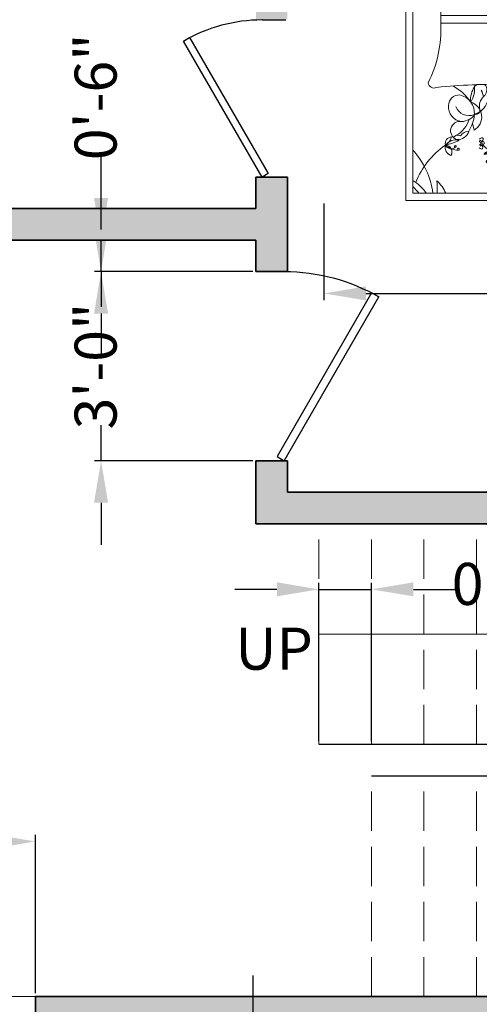
# Model space of a CAD drawing. Units: inches. Extents: x 2073 to 2646, y 2372 to 3017.
# Tile 5 of 8: x 2340 to 2428, y 2686 to 2874. Entities that reach past the tile are written whole.
import ezdxf

# ---------------------------------------------------------------- set-up
doc = ezdxf.new("R2010")
doc.units = ezdxf.units.IN
doc.linetypes.add('DASH', pattern=[0.35, 0.25, -0.1])
for name, color, linetype, lineweight in [('A-ANNO-DIMS', 2, 'Continuous', 18), ('A-ANNO-SYMB', 7, 'Continuous', 18), ('A-ANNO-TEXT', 7, 'Continuous', 25), ('A-DOOR', 3, 'Continuous', 25), ('A-FLOR-STRS', 7, 'Continuous', 25), ('A-FLOR-STRS-HIDN', 7, 'DASH', 18), ('A-FURN', 8, 'Continuous', 18), ('A-WALL', 7, 'Continuous', 35), ('A-WALL-OVHD', 7, 'DASH', 18), ('A-WALL-PATT', 30, 'Continuous', 13)]:
    doc.layers.add(name, color=color, linetype=linetype, lineweight=lineweight)
doc.styles.get("Standard").update_dxf_attribs({"font": 'arial.ttf'})
doc.dimstyles.new('ISO-25', dxfattribs={"dimtxt": 8, "dimasz": 8, "dimexe": 1.25, "dimexo": 0.625, "dimtad": 0, "dimdec": 1, "dimlunit": 4, "dimtxsty": 'Standard', "dimcen": 2.5, "dimadec": 0, "dimazin": 0, "dimtfac": 1, "dimtdec": 1, "dimtmove": 0, "dimatfit": 3, "dimfxl": 1, "dimarcsym": 0})

# ---------------------------------------------------------------- blocks, each defined once
blk = doc.blocks.new('bed')
at = {"color": 0}
for p, q in [((2249.53, 3172.75), (2367.64, 3172.75)), ((2273.15, 3172.75), (2273.15, 3140.33)), ((2261.34, 3155.19), (2261.34, 3170.62)), ((2344.02, 3171.23), (2273.15, 3171.23)), ((2355.83, 3155.19), (2355.83, 3170.62)), ((2269.06, 3162.9), (2253.62, 3162.9)), ((2348.11, 3162.9), (2363.55, 3162.9)), ((2273.15, 3154.08), (2344.02, 3154.08)), ((2289.56, 3150.57), (2302.44, 3154.08)), ((2305.6, 3154.08), (2299.13, 3145.07)), ((2280.95, 3147.46), (2289.56, 3150.57)), ((2343.7, 3149.18), (2301.65, 3148.59)), ((2276.4, 3144.12), (2280.95, 3147.46)), ((2343.66, 3147.96), (2300.77, 3147.36)), ((2272.09, 3139.1), (2276.4, 3144.12)), ((2299.13, 3145.07), (2296.5, 3138.14)), ((2343.59, 3144.24), (2298.75, 3144.07)), ((2343.6, 3143.03), (2298.28, 3142.85)), ((2273.05, 3138.14), (2272.09, 3139.1)), ((2277.84, 3138.62), (2273.05, 3138.14)), ((2283.82, 3138.14), (2277.84, 3138.62)), ((2289.08, 3137.42), (2283.82, 3138.14)), ((2296.5, 3138.14), (2296.02, 3135.03)), ((2292.19, 3135.99), (2289.08, 3137.42)), ((2296.02, 3135.03), (2292.19, 3135.99)), ((2265.12, 3114.85), (2271.8, 3114.85)), ((2265.12, 3072.3), (2265.12, 3114.85)), ((2344.68, 3114.85), (2351.23, 3114.85)), ((2351.23, 3114.85), (2351.23, 3072.3)), ((2271.8, 3113.48), (2266.49, 3113.48)), ((2266.49, 3113.48), (2266.49, 3073.67)), ((2349.86, 3113.48), (2344.65, 3113.48)), ((2349.86, 3073.67), (2349.86, 3113.48)), ((2344.56, 3107.48), (2271.79, 3107.48)), ((2344.67, 3106.01), (2271.79, 3106.01)), ((2332.56, 3094.41), (2284.61, 3094.41)), ((2278.13, 3085.65), (2277.87, 3086.98)), ((2286.38, 3085.65), (2286.64, 3086.98)), ((2329.96, 3085.65), (2329.7, 3086.98)), ((2338.22, 3085.65), (2338.48, 3086.98)), ((2266.49, 3073.67), (2349.86, 3073.67)), ((2351.23, 3072.3), (2265.12, 3072.3))]:
    blk.add_line(p, q, dxfattribs=at)
for points in [[(2273.15, 3153.06), (2249.53, 3153.06), (2249.53, 3172.75)], [(2344.02, 3172.75), (2344.02, 3153.06), (2367.64, 3153.06), (2367.64, 3172.75)], [(2261.34, 3162.9), (2262.72, 3165.29)], [(2355.83, 3162.9), (2354.45, 3165.29)], [(2261.34, 3162.9), (2262.72, 3160.52)], [(2355.83, 3162.9), (2354.45, 3160.52)]]:
    blk.add_lwpolyline(points, dxfattribs=at)
for points in [[(2279.94, 3169.8, 0.074897), (2280.08, 3162.09, -0.472817)], [(2337.23, 3169.8, -0.074897), (2337.09, 3162.09, 0.472817)], [(2308.03, 3161.66, 0.14099), (2308.27, 3169.53, 0.235245)], [(2313.08, 3161.66, -0.14099), (2312.84, 3169.53, -0.235245)], [(2271.85, 3128.28, 0.001242), (2271.79, 3105.87, -0.127202), (2269.42, 3094.7)], [(2344.52, 3108.41, 0.056112), (2345.38, 3101.91, 0.095341), (2347.04, 3095.66)]]:
    blk.add_lwpolyline(points, format="xyb", dxfattribs=at)
for centre, radius in [((2261.34, 3162.9), 5.51), ((2355.83, 3162.9), 5.51), ((2261.34, 3162.9), 2.76), ((2355.83, 3162.9), 2.76), ((2284.95, 3081.37), 0.301), ((2331.4, 3081.37), 0.301), ((2282.98, 3078.2), 0.301), ((2333.36, 3078.2), 0.301)]:
    blk.add_circle(centre, radius, dxfattribs=at)
for centre, radius, start, end in [((2345.04, 4293.82), 1125.9, 266.68521, 267.14978), ((2296.12, 3127.06), 42.84, 82.2196, 99.497), ((2323.22, 3149.14), 20.76, 76.3427, 101.1841), ((2272.13, 4293.82), 1125.9, 272.85022, 273.31479), ((2305.17, 3148.71), 21.05, 81.5249, 103.96), ((2314.46, 3163.91), 5.84, 63.3437, 106.1026), ((2294.98, 3158.99), 15.22, 155.1316, 191.7583), ((2322.19, 3158.99), 15.22, 348.2417, 24.8684), ((2294.11, 3157.71), 14.47, 354.0129, 15.8293), ((2327, 3157.71), 14.47, 164.1707, 185.9871), ((2284.15, 3171.19), 15.83, 255.1039, 281.0369), ((2292.48, 3182.44), 27.45, 258.0397, 289.2615), ((2303.6, 3176.44), 20.83, 259.8617, 283.6238), ((2315.25, 3161.88), 6.26, 245.0183, 288.5407), ((2326.19, 3170.02), 15.03, 243.8761, 286.1746), ((2333.02, 3171.19), 15.83, 258.9631, 284.8961), ((2555.75, 3139.65), 212.22, 176.1, 180.9282), ((2163.8, 3136.16), 108.33, 355.8294, 1.553), ((2274.12, 3180.92), 44.58, 267.4519, 281.3392), ((2284.77, 3127.79), 9.61, 66.2616, 101.3392), ((2304.22, 3179.66), 45.8, 250.1194, 259.3383), ((2620.36, 3131.93), 276.84, 179.1145, 184.8735), ((2295.75, 3134.94), 0.285, 268.8623, 19.7536), ((2346.15, 3095.06), 1.08, 246.5219, 33.8264), ((2270.51, 3094.78), 1.09, 183.98, 297.3412), ((2283.2, 2971.46), 122.95, 89.3433, 95.6887), ((2270.05, 3086.09), 8.94, 33.6671, 63.2997), ((2282.03, 3091.41), 4.56, 145.785, 184.7304), ((2273.33, 3093.53), 4.89, 328.8218, 9.1554), ((2279.39, 3093.1), 1.42, 120.0293, 142.325), ((2277.12, 3092.26), 3.76, 289.2822, 29.1751), ((2276.55, 3091.58), 3.4, 7.436, 29.9149), ((2278.79, 3093.38), 1.77, 311.5653, 23.8354), ((2279.39, 3093.1), 1.42, 44.4517, 63.558), ((2287.39, 3092.26), 3.76, 150.8249, 250.7178), ((2285.72, 3093.38), 1.77, 156.1646, 228.4347), ((2285.12, 3093.1), 1.42, 113.229, 135.5483), ((2287.96, 3091.58), 3.4, 150.0851, 172.564), ((2285.12, 3093.1), 1.42, 37.675, 66.7144), ((2282.48, 3091.41), 4.56, 355.2696, 34.215), ((2291.18, 3093.53), 4.89, 169.7133, 211.1782), ((2294.46, 3086.09), 8.94, 111.4941, 146.3329), ((2321.89, 3086.09), 8.94, 33.6671, 68.5059), ((2333.87, 3091.41), 4.56, 145.785, 184.7304), ((2325.17, 3093.53), 4.89, 328.8218, 10.2867), ((2331.23, 3093.1), 1.42, 113.2856, 142.325), ((2328.96, 3092.26), 3.76, 289.2822, 29.1751), ((2328.39, 3091.58), 3.4, 7.436, 29.9149), ((2331.23, 3093.1), 1.42, 44.4517, 66.7144), ((2330.63, 3093.38), 1.77, 311.5653, 23.8354), ((2336.18, 2979.53), 114.93, 85.2402, 91.8035), ((2339.23, 3092.26), 3.76, 150.8249, 250.7178), ((2337.56, 3093.38), 1.77, 156.1646, 228.4347), ((2336.96, 3093.1), 1.42, 106.6343, 135.5483), ((2339.8, 3091.58), 3.4, 150.0851, 172.564), ((2336.96, 3093.1), 1.42, 37.675, 72.5814), ((2334.32, 3091.41), 4.56, 355.2696, 34.215), ((2343.02, 3093.53), 4.89, 169.249, 211.1782), ((2346.3, 3086.09), 8.94, 113.6453, 146.3329), ((2275.26, 3090.38), 1.99, 84.4856, 181.0538), ((2274.65, 3088.91), 3.55, 355.2933, 76.921), ((2281.57, 3090.25), 2.42, 131.5653, 195.1471), ((2282.94, 3090.25), 2.42, 344.8529, 48.4347), ((2289.86, 3088.91), 3.55, 103.079, 184.7067), ((2289.25, 3090.38), 1.99, 358.9462, 95.5144), ((2327.09, 3090.38), 1.99, 84.4856, 181.0538), ((2326.48, 3088.91), 3.55, 355.2933, 76.921), ((2333.4, 3090.25), 2.42, 131.5653, 195.1471), ((2334.78, 3090.25), 2.42, 344.8529, 48.4347), ((2341.7, 3088.91), 3.55, 103.079, 184.7067), ((2341.09, 3090.38), 1.99, 358.9462, 95.5144), ((2276.08, 3090.1), 2.82, 174.9449, 262.8857), ((2277.18, 3091.17), 2.74, 201.5819, 291.4221), ((2276.66, 3088.19), 2.94, 299.9085, 73.1337), ((2278.52, 3089.43), 0.733, 257.3041, 15.1471), ((2287.85, 3088.19), 2.94, 106.8663, 240.0915), ((2285.99, 3089.43), 0.733, 164.8529, 282.6959), ((2287.32, 3091.17), 2.74, 248.5779, 338.4181), ((2288.43, 3090.1), 2.82, 277.1143, 5.0551), ((2327.91, 3090.1), 2.82, 174.9449, 262.8857), ((2329.02, 3091.17), 2.74, 201.5819, 291.4221), ((2328.5, 3088.19), 2.94, 299.9085, 73.1337), ((2330.36, 3089.43), 0.733, 257.3041, 15.1471), ((2339.68, 3088.19), 2.94, 106.8663, 240.0915), ((2337.82, 3089.43), 0.733, 164.8529, 282.6959), ((2339.16, 3091.17), 2.74, 248.5779, 338.4181), ((2340.27, 3090.1), 2.82, 277.1143, 5.0551), ((2275.43, 3085.55), 1.77, 80.264, 250.8688), ((2271.91, 3089.45), 5.58, 301.2614, 341.7045), ((2275.58, 3090.72), 3.43, 272.3591, 324.0401), ((2271.86, 3089), 6.34, 326.2883, 356.5076), ((2282.03, 3091.41), 4.56, 212.7011, 216.3445), ((2282.59, 3088.31), 0.228, 102.7051, 280.4384), ((2282.57, 3088.45), 0.37, 280.4384, 100.4136), ((2282.48, 3091.41), 4.56, 323.6555, 327.2989), ((2288.92, 3090.72), 3.43, 215.9599, 267.6409), ((2292.65, 3089), 6.34, 183.4924, 213.7117), ((2292.6, 3089.45), 5.58, 198.2955, 238.7386), ((2289.08, 3085.55), 1.77, 289.1312, 99.736), ((2309.53, 3086.61), 1.28, 63.0274, 163.8037), ((2308.24, 3089.6), 2.63, 271.4585, 315.3727), ((2310.75, 3086.61), 1.28, 16.1963, 116.9726), ((2312.05, 3089.6), 2.63, 224.6273, 268.5415), ((2327.26, 3085.55), 1.77, 80.264, 250.8688), ((2323.75, 3089.45), 5.58, 301.2614, 341.7045), ((2327.42, 3090.72), 3.43, 272.3591, 324.0401), ((2323.7, 3089), 6.34, 326.2883, 356.5076), ((2333.87, 3091.41), 4.56, 212.7011, 216.3445), ((2333.78, 3088.45), 0.37, 79.5864, 259.5616), ((2333.75, 3088.31), 0.228, 259.5616, 77.2949), ((2334.32, 3091.41), 4.56, 323.6555, 327.2989), ((2340.76, 3090.72), 3.43, 215.9599, 267.6409), ((2344.49, 3089), 6.34, 183.4924, 213.7117), ((2344.44, 3089.45), 5.58, 198.2955, 238.7386), ((2340.92, 3085.55), 1.77, 289.1312, 99.736), ((2275, 3086.08), 2.21, 265.969, 344.3045), ((2277.38, 3083.14), 2.36, 96.1662, 141.5825), ((2279.99, 3086.89), 1.9, 308.2101, 316.3071), ((2281.16, 3085.65), 0.567, 278.3432, 4.2869), ((2280.84, 3086.14), 0.99, 300.656, 332.6341), ((2281.59, 3085.49), 0.241, 55.7657, 157.4417), ((2290.78, 3082.37), 9.78, 153.0032, 159.8941), ((2281.96, 3085.71), 0.241, 84.3784, 186.0543), ((2281.74, 3086.68), 0.99, 269.1859, 301.164), ((2282.03, 3086.17), 0.567, 237.5332, 323.4768), ((2281.48, 3087.78), 1.9, 285.5129, 293.6099), ((2282.72, 3085.65), 0.62, 87.3579, 140.4944), ((2281.28, 3087.43), 1.87, 301.164, 321.5612), ((2279.77, 3087.76), 3.33, 324.6898, 333.4936), ((2287.12, 3083.14), 2.36, 38.4175, 83.8338), ((2289.51, 3086.08), 2.21, 195.6955, 274.031), ((2309.5, 3071.59), 15.42, 94.4623, 172.255), ((2309.57, 3085.82), 1.71, 137.7873, 219.1145), ((2307.63, 3085.87), 1.29, 298.5391, 58.3627), ((2309.31, 3084.75), 2.44, 45.5411, 114.3101), ((2311.53, 3097.27), 10.79, 252.593, 267.2582), ((2309.56, 3086.92), 1.26, 177.7585, 283.852), ((2311.99, 3088.23), 3.9, 198.9159, 238.011), ((2310.98, 3084.75), 2.44, 65.6899, 134.4589), ((2308.75, 3097.27), 10.79, 272.7418, 287.407), ((2309.83, 3085.86), 0.167, 283.852, 219.9245), ((2310.44, 3085.92), 0.101, 320.1909, 256.0209), ((2308.29, 3088.23), 3.9, 301.989, 341.0841), ((2310.72, 3086.92), 1.26, 256.148, 2.2415), ((2312.66, 3085.87), 1.29, 121.6373, 241.4609), ((2310.71, 3085.82), 1.71, 320.8855, 42.2127), ((2310.28, 3075.15), 11.94, 352.8636, 81.8197), ((2326.84, 3086.08), 2.21, 265.969, 344.3045), ((2329.22, 3083.14), 2.36, 96.1662, 141.5825), ((2335.06, 3087.43), 1.87, 218.4388, 238.836), ((2333.63, 3085.65), 0.62, 39.5056, 92.6421), ((2336.58, 3087.76), 3.33, 206.5064, 215.3102), ((2334.32, 3086.17), 0.567, 216.5232, 302.4668), ((2334.61, 3086.68), 0.99, 238.836, 270.8141), ((2334.87, 3087.78), 1.9, 246.3901, 254.4871), ((2325.57, 3082.37), 9.78, 20.1059, 26.9968), ((2334.38, 3085.71), 0.241, 353.9457, 95.6216), ((2334.76, 3085.49), 0.241, 22.5583, 124.2343), ((2335.19, 3085.65), 0.567, 175.7131, 261.6568), ((2335.5, 3086.14), 0.99, 207.3659, 239.344), ((2336.35, 3086.89), 1.9, 223.6929, 231.7899), ((2341.35, 3086.08), 2.21, 195.6955, 274.031), ((2338.96, 3083.14), 2.36, 38.4175, 83.8338), ((2273.92, 3083.1), 1.28, 92.9516, 193.728), ((2271.31, 3085.04), 2.63, 301.3827, 345.2969), ((2274.66, 3081.37), 2.44, 75.4653, 144.2343), ((2270.34, 3093.33), 10.79, 282.5173, 297.1824), ((2275.06, 3083.63), 1.09, 63.9755, 143.2681), ((2279.54, 3083.62), 0.502, 101.5637, 142.6358), ((2279.47, 3083.44), 0.287, 91.1081, 181.8675), ((2279.13, 3084.01), 0.723, 288.7263, 352.5032), ((2279.63, 3083.98), 0.232, 345.2356, 144.9248), ((2281.29, 3084.79), 0.62, 101.3256, 154.4621), ((2280.4, 3086.9), 1.87, 280.2588, 300.656), ((2280.83, 3088.39), 3.33, 268.3264, 277.1302), ((2290.78, 3082.37), 9.78, 163.5842, 183.8277), ((2289.45, 3083.63), 1.09, 36.7319, 116.0245), ((2289.85, 3081.37), 2.44, 35.7657, 104.5347), ((2294.17, 3093.33), 10.79, 242.8176, 257.4827), ((2290.59, 3083.1), 1.28, 346.272, 87.0484), ((2293.2, 3085.04), 2.63, 194.7031, 238.6173), ((2310.03, 3085.09), 0.192, 238.011, 71.5592), ((2310.06, 3085.18), 0.093, 71.5592, 188.0167), ((2310.25, 3085.09), 0.192, 108.4408, 301.989), ((2310.22, 3085.18), 0.093, 351.9833, 108.4408), ((2325.76, 3083.1), 1.28, 92.9516, 193.728), ((2323.15, 3085.04), 2.63, 301.3827, 345.2969), ((2326.5, 3081.37), 2.44, 75.4653, 144.2343), ((2322.18, 3093.33), 10.79, 282.5173, 297.1824), ((2326.9, 3083.63), 1.09, 63.9755, 143.2681), ((2325.57, 3082.37), 9.78, 356.1723, 16.4158), ((2335.95, 3086.9), 1.87, 239.344, 259.7412), ((2335.52, 3088.39), 3.33, 262.8698, 271.6736), ((2335.06, 3084.79), 0.62, 25.5379, 78.6744), ((2336.72, 3083.98), 0.232, 35.0752, 194.7644), ((2337.21, 3084.01), 0.723, 187.4968, 251.2737), ((2336.88, 3083.44), 0.287, 358.1325, 88.8919), ((2336.81, 3083.62), 0.502, 37.3642, 78.4363), ((2341.29, 3083.63), 1.09, 36.7319, 116.0245), ((2341.69, 3081.37), 2.44, 35.7657, 104.5347), ((2346, 3093.33), 10.79, 242.8176, 257.4827), ((2345.04, 3085.04), 2.63, 194.7031, 238.6173), ((2342.42, 3083.1), 1.28, 346.272, 87.0484), ((2255.01, 3071.59), 15.42, 7.745, 41.8856), ((2281.39, 3070.07), 15.42, 124.3865, 158.5908), ((2274.35, 3082.43), 1.71, 167.7115, 249.0387), ((2272.64, 3081.51), 1.29, 328.4633, 88.2869), ((2275.25, 3085.73), 3.9, 228.8402, 267.9352), ((2273.8, 3083.38), 1.26, 207.6827, 313.7762), ((2274.56, 3082.59), 0.167, 313.7762, 249.7183), ((2275.1, 3082.12), 0.093, 101.4834, 217.9409), ((2275.12, 3082.03), 0.192, 267.9352, 101.4834), ((2279.12, 3083.15), 0.301, 273.2768, 86.7232), ((2279.53, 3082.6), 0.497, 217.7621, 259.0403), ((2280.07, 3083.26), 0.913, 203.4276, 227.6104), ((2279.78, 3082.86), 0.622, 80.3487, 133.6538), ((2279.66, 3083.37), 0.492, 229.7889, 317.6792), ((2279.11, 3082.33), 0.699, 355.053, 68.3618), ((2279.66, 3082.21), 0.985, 83.0852, 105.7171), ((2279.58, 3082.29), 0.231, 232.4737, 355.053), ((2272.84, 3074.04), 11.21, 43.1541, 52.0459), ((2279.84, 3083.22), 0.259, 317.6792, 80.3487), ((2280.45, 3081.67), 0.567, 278.3432, 4.2869), ((2280.14, 3082.17), 0.99, 300.656, 332.6341), ((2280.88, 3081.52), 0.241, 55.7657, 157.4417), ((2285.91, 3082.12), 4.9, 184.756, 209.2041), ((2292.97, 3092.56), 16.14, 222.2412, 232.1744), ((2282.65, 3081.81), 1.37, 304.5369, 16.3699), ((2284.55, 3081.43), 0.97, 127.3105, 187.9252), ((2283.22, 3081.54), 0.996, 355.0106, 41.658), ((2284.62, 3081.78), 0.41, 126.1046, 271.4281), ((2284.57, 3081.9), 0.295, 353.7526, 131.7054), ((2284.3, 3081.55), 0.414, 0.0645, 61.1507), ((2284.39, 3081.9), 0.473, 311.8413, 355.7877), ((2285.37, 3081.83), 0.502, 101.5637, 176.365), ((2285.3, 3081.65), 0.287, 91.1081, 181.8675), ((2285.61, 3081.07), 0.622, 80.3487, 133.6538), ((2284.96, 3082.22), 0.723, 288.7263, 352.5032), ((2285.46, 3082.19), 0.232, 345.2356, 144.9248), ((2285.67, 3081.43), 0.259, 317.6792, 80.3487), ((2289.39, 3082.03), 0.192, 78.5166, 272.0648), ((2289.26, 3085.73), 3.9, 272.0648, 311.1598), ((2289.41, 3082.12), 0.093, 322.0591, 78.5166), ((2290.71, 3083.38), 1.26, 226.2238, 332.3173), ((2289.97, 3082.66), 0.101, 290.2667, 226.2271), ((2291.87, 3081.51), 1.29, 91.7131, 211.5367), ((2290.16, 3082.43), 1.71, 290.9613, 12.2885), ((2283.12, 3070.07), 15.42, 21.4092, 55.6135), ((2333.23, 3070.07), 15.42, 124.3865, 158.5908), ((2326.19, 3082.43), 1.71, 167.7115, 249.0387), ((2325.64, 3083.38), 1.26, 207.6827, 313.7762), ((2327.09, 3085.73), 3.9, 228.8402, 267.9352), ((2324.48, 3081.51), 1.29, 328.4633, 88.2869), ((2326.39, 3082.59), 0.167, 313.7762, 249.7183), ((2326.93, 3082.12), 0.093, 101.4834, 217.9409), ((2326.95, 3082.03), 0.192, 267.9352, 101.4834), ((2330.68, 3081.43), 0.259, 99.6513, 222.3208), ((2330.74, 3081.07), 0.622, 46.3462, 99.6513), ((2330.89, 3082.19), 0.232, 35.0752, 194.7644), ((2331.38, 3082.22), 0.723, 187.4968, 251.2737), ((2331.05, 3081.65), 0.287, 358.1325, 88.8919), ((2330.98, 3081.83), 0.502, 3.635, 78.4363), ((2331.77, 3081.9), 0.295, 48.2946, 186.2474), ((2331.95, 3081.9), 0.473, 184.2123, 228.1587), ((2332.05, 3081.55), 0.414, 118.8493, 179.9355), ((2331.73, 3081.78), 0.41, 268.5719, 53.8954), ((2333.13, 3081.54), 0.996, 138.342, 184.9894), ((2333.7, 3081.81), 1.37, 163.6301, 235.4631), ((2331.79, 3081.43), 0.97, 352.0748, 52.6895), ((2323.38, 3092.56), 16.14, 307.8256, 317.7588), ((2330.44, 3082.12), 4.9, 330.7959, 355.244), ((2343.51, 3074.04), 11.21, 127.9541, 136.8459), ((2335.46, 3081.52), 0.241, 22.5583, 124.2343), ((2335.89, 3081.67), 0.567, 175.7131, 261.6568), ((2336.21, 3082.17), 0.99, 207.3659, 239.344), ((2336.51, 3083.22), 0.259, 99.6513, 222.3208), ((2336.68, 3083.37), 0.492, 222.3208, 310.2111), ((2336.57, 3082.86), 0.622, 46.3462, 99.6513), ((2337.24, 3082.33), 0.699, 111.6382, 184.947), ((2336.77, 3082.29), 0.231, 184.947, 307.5263), ((2336.69, 3082.21), 0.985, 74.2829, 96.9148), ((2336.28, 3083.26), 0.913, 312.3896, 336.5724), ((2336.82, 3082.6), 0.497, 280.9597, 322.2379), ((2337.23, 3083.15), 0.301, 93.2768, 266.7232), ((2341.23, 3082.03), 0.192, 78.5166, 272.0648), ((2341.1, 3085.73), 3.9, 272.0648, 311.1598), ((2341.25, 3082.12), 0.093, 322.0591, 78.5166), ((2342.55, 3083.38), 1.26, 226.2238, 332.3173), ((2341.81, 3082.66), 0.101, 290.2667, 226.2271), ((2343.7, 3081.51), 1.29, 91.7131, 211.5367), ((2341.99, 3082.43), 1.71, 290.9613, 12.2885), ((2334.95, 3070.07), 15.42, 21.4092, 55.6135), ((2361.34, 3071.59), 15.42, 138.1144, 172.255), ((2280.59, 3080.82), 0.62, 101.3256, 154.4621), ((2279.69, 3082.92), 1.87, 280.2588, 300.656), ((2280.12, 3084.42), 3.33, 268.3264, 277.1302), ((2279.29, 3082.92), 1.9, 308.2101, 316.3071), ((2280.79, 3079.73), 0.336, 146.8636, 236.9021), ((2285.53, 3087.13), 8.79, 235.1882, 238.8844), ((2281.37, 3080.22), 0.909, 199.4799, 267.6828), ((2286.41, 3075.61), 5.88, 120.544, 139.818), ((2283.06, 3078.85), 0.97, 70.0041, 130.6188), ((2283.38, 3081.51), 0.833, 272.8499, 356.1226), ((2282.79, 3081.18), 0.807, 321.7607, 7.9252), ((2282.96, 3080.02), 0.807, 8.7227, 54.8872), ((2283, 3079.38), 1.37, 0.278, 72.111), ((2283.62, 3079.88), 0.833, 20.5253, 88.5375), ((2284.72, 3080.29), 0.97, 188.7227, 249.3375), ((2284.32, 3080.8), 0.298, 148.0499, 225.6268), ((2286.41, 3075.61), 5.88, 113.0501, 113.8477), ((2284.87, 3080.46), 0.948, 104.7558, 148.0499), ((2284.34, 3081.14), 0.594, 247.4086, 351.4386), ((2283.47, 3079.81), 0.996, 334.9899, 21.6373), ((2284.51, 3081.11), 0.199, 262.906, 7.132), ((2285.36, 3080.81), 0.497, 151.2196, 259.0403), ((2285.9, 3081.47), 0.913, 203.4276, 227.6104), ((2285.5, 3081.59), 0.492, 229.7889, 317.6792), ((2284.94, 3080.54), 0.699, 355.053, 68.3618), ((2285.49, 3080.43), 0.985, 83.0852, 105.7171), ((2285.41, 3080.5), 0.231, 232.4737, 355.053), ((2286.41, 3075.61), 5.88, 87.1071, 94.7585), ((2329.94, 3075.61), 5.88, 85.2415, 92.8929), ((2330.85, 3081.59), 0.492, 222.3208, 310.2111), ((2331.41, 3080.54), 0.699, 111.6382, 184.947), ((2330.94, 3080.5), 0.231, 184.947, 307.5263), ((2330.86, 3080.43), 0.985, 74.2829, 96.9148), ((2330.45, 3081.47), 0.913, 312.3896, 336.5724), ((2330.99, 3080.81), 0.497, 280.9597, 28.7804), ((2332.01, 3081.14), 0.594, 188.5614, 292.5914), ((2331.84, 3081.11), 0.199, 172.868, 277.094), ((2331.48, 3080.46), 0.948, 31.9501, 75.2442), ((2332.87, 3079.81), 0.996, 158.3627, 205.0101), ((2332.73, 3079.88), 0.833, 91.4625, 159.4747), ((2333.34, 3079.38), 1.37, 107.889, 179.722), ((2331.63, 3080.29), 0.97, 290.6625, 351.2773), ((2332.97, 3081.51), 0.833, 183.8774, 267.1501), ((2329.94, 3075.61), 5.88, 66.1523, 66.9499), ((2332.03, 3080.8), 0.298, 314.3732, 31.9501), ((2333.39, 3080.02), 0.807, 125.1128, 171.2773), ((2333.55, 3081.18), 0.807, 172.0748, 218.2393), ((2329.94, 3075.61), 5.88, 40.182, 59.456), ((2333.29, 3078.85), 0.97, 49.3812, 109.9959), ((2334.98, 3080.22), 0.909, 272.3172, 340.5201), ((2330.82, 3087.13), 8.79, 301.1156, 304.8118), ((2337.06, 3082.92), 1.9, 223.6929, 231.7899), ((2336.65, 3082.92), 1.87, 239.344, 259.7412), ((2335.55, 3079.73), 0.336, 303.0979, 33.1364), ((2336.22, 3084.42), 3.33, 262.8698, 271.6736), ((2335.76, 3080.82), 0.62, 25.5379, 78.6744), ((2281.27, 3079.88), 0.783, 212.8155, 277.3992), ((2280.81, 3079.35), 0.909, 266.9701, 338.2913), ((2276.02, 3085.84), 8.79, 302.6784, 306.3746), ((2281.04, 3078.63), 0.336, 214.3538, 304.3923), ((2281.17, 3079.91), 0.348, 238.8844, 314.2646), ((2281.09, 3079.13), 0.783, 280.3057, 17.1958), ((2281.03, 3079.05), 0.348, 306.3746, 21.7548), ((2281.59, 3079.27), 0.262, 19.3605, 201.7548), ((2281.59, 3079.47), 0.262, 311.8703, 134.2646), ((2286.53, 3077.08), 5.24, 153.7819, 158.2913), ((2282.36, 3080.66), 1.37, 247.2305, 319.0635), ((2281.9, 3080.2), 0.807, 264.4544, 310.6188), ((2285.91, 3082.12), 4.9, 214.0033, 222.4917), ((2282.49, 3079.88), 0.833, 218.3208, 298.8162), ((2282.9, 3077.29), 0.948, 104.7558, 148.0499), ((2282.65, 3078.61), 0.41, 126.1046, 271.4281), ((2282.61, 3078.72), 0.295, 353.7526, 131.7054), ((2282.54, 3077.94), 0.199, 262.906, 7.132), ((2282.33, 3078.37), 0.414, 0.0645, 61.1507), ((2282.43, 3078.73), 0.473, 311.8413, 355.7877), ((2282.43, 3080.03), 0.996, 297.7043, 344.3516), ((2283.4, 3078.66), 0.502, 101.5637, 176.365), ((2283.33, 3078.48), 0.287, 91.1081, 181.8675), ((2283.93, 3078.3), 0.913, 203.4276, 227.6104), ((2283.64, 3077.9), 0.622, 80.3487, 133.6538), ((2283.53, 3078.42), 0.492, 229.7889, 317.6792), ((2283, 3079.05), 0.723, 288.7263, 352.5032), ((2282.97, 3077.37), 0.699, 355.053, 68.3618), ((2283.52, 3077.26), 0.985, 83.0852, 105.7171), ((2283.49, 3079.02), 0.232, 345.2356, 144.9248), ((2283.7, 3078.26), 0.259, 317.6792, 80.3487), ((2308.32, 3063.33), 15.42, 94.4623, 117.4146), ((2308.39, 3077.56), 1.71, 137.7873, 219.1145), ((2306.45, 3077.61), 1.29, 298.5391, 58.3627), ((2308.35, 3078.35), 1.28, 63.0274, 163.8037), ((2307.06, 3081.34), 2.63, 271.4585, 315.3727), ((2308.13, 3076.49), 2.44, 45.5411, 114.3101), ((2310.81, 3079.97), 3.9, 198.9159, 238.011), ((2310.35, 3089), 10.79, 252.593, 267.2582), ((2308.38, 3078.66), 1.26, 177.7585, 283.852), ((2312.16, 3076.49), 2.44, 65.6899, 134.4589), ((2309.93, 3089), 10.79, 272.7418, 287.407), ((2311.93, 3078.35), 1.28, 16.1963, 116.9726), ((2313.23, 3081.34), 2.63, 224.6273, 268.5415), ((2309.47, 3079.97), 3.9, 301.989, 341.0841), ((2311.9, 3078.66), 1.26, 256.148, 2.2415), ((2313.84, 3077.61), 1.29, 121.6373, 241.4609), ((2311.89, 3077.56), 1.71, 320.8855, 42.2127), ((2311.96, 3063.33), 15.42, 62.5854, 85.5377), ((2332.65, 3078.26), 0.259, 99.6513, 222.3208), ((2332.82, 3078.42), 0.492, 222.3208, 310.2111), ((2332.71, 3077.9), 0.622, 46.3462, 99.6513), ((2332.86, 3079.02), 0.232, 35.0752, 194.7644), ((2333.35, 3079.05), 0.723, 187.4968, 251.2737), ((2333.37, 3077.37), 0.699, 111.6382, 184.947), ((2332.83, 3077.26), 0.985, 74.2829, 96.9148), ((2333.99, 3080.66), 1.37, 220.9365, 292.7695), ((2333.91, 3080.03), 0.996, 195.6484, 242.2957), ((2333.01, 3078.48), 0.287, 358.1325, 88.8919), ((2332.42, 3078.3), 0.913, 312.3896, 336.5724), ((2332.95, 3078.66), 0.502, 3.635, 78.4363), ((2333.85, 3079.88), 0.833, 241.1838, 321.6792), ((2333.74, 3078.72), 0.295, 48.2946, 186.2474), ((2333.92, 3078.73), 0.473, 184.2123, 228.1587), ((2334.02, 3078.37), 0.414, 118.8493, 179.9355), ((2333.81, 3077.94), 0.199, 172.868, 277.094), ((2333.7, 3078.61), 0.41, 268.5719, 53.8954), ((2333.44, 3077.29), 0.948, 31.9501, 75.2442), ((2334.44, 3080.2), 0.807, 229.3812, 275.5456), ((2330.44, 3082.12), 4.9, 317.5083, 325.9967), ((2335.25, 3079.13), 0.783, 162.8042, 259.6943), ((2334.75, 3079.47), 0.262, 45.7354, 228.1297), ((2334.75, 3079.27), 0.262, 338.2452, 160.6395), ((2329.82, 3077.08), 5.24, 21.7087, 26.2181), ((2335.53, 3079.35), 0.909, 201.7087, 273.0299), ((2335.18, 3079.91), 0.348, 225.7354, 301.1156), ((2335.32, 3079.05), 0.348, 158.2452, 233.6254), ((2335.08, 3079.88), 0.783, 262.6008, 327.1845), ((2340.32, 3085.84), 8.79, 233.6254, 237.3216), ((2335.3, 3078.63), 0.336, 235.6077, 325.6462), ((2282.35, 3077.63), 0.298, 148.0499, 225.6268), ((2282.37, 3077.97), 0.594, 247.4086, 351.4386), ((2283.39, 3077.64), 0.497, 151.2196, 259.0403), ((2283.44, 3077.33), 0.231, 232.4737, 355.053), ((2301.77, 3069.53), 7.52, 91.272, 146.5383), ((2304.47, 3068.13), 9.37, 107.8504, 143.6964), ((2309.39, 3065.49), 13.93, 124.0123, 144.053), ((2308.65, 3077.6), 0.167, 283.852, 219.9245), ((2308.85, 3076.83), 0.192, 238.011, 71.5592), ((2308.88, 3076.92), 0.093, 71.5592, 188.0167), ((2311.44, 3076.83), 0.192, 108.4408, 301.989), ((2311.4, 3076.92), 0.093, 351.9833, 108.4408), ((2311.62, 3077.66), 0.101, 320.1909, 256.0209), ((2311.82, 3076.24), 6.91, 338.117, 6.6195), ((2318.16, 3074.32), 2.77, 346.3898, 79.0739), ((2316.08, 3074.7), 3.5, 342.8609, 41.9049), ((2332.91, 3077.33), 0.231, 184.947, 307.5263), ((2332.95, 3077.64), 0.497, 280.9597, 28.7804), ((2333.98, 3077.97), 0.594, 188.5614, 292.5914), ((2334, 3077.63), 0.298, 314.3732, 31.9501), ((2262.74, 3069.53), 7.52, 33.4617, 60.1116), ((2260.04, 3068.13), 9.37, 36.3036, 46.4814), ((2266.95, 3071.27), 6.27, 22.5547, 48.9546), ((2249.77, 3074.64), 21.34, 357.4081, 3.6519), ((2297.56, 3071.27), 6.27, 131.0454, 157.4453), ((2314.73, 3074.64), 21.34, 176.3481, 182.5919), ((2301.61, 3074.64), 21.34, 357.4081, 3.6519), ((2318.79, 3071.27), 6.27, 22.5547, 48.9546), ((2349.39, 3071.27), 6.27, 131.0454, 157.4453), ((2366.57, 3074.64), 21.34, 176.3481, 182.5919), ((2353.6, 3069.53), 7.52, 119.8884, 146.5383), ((2356.31, 3068.13), 9.37, 133.5186, 143.6964), ((2304.01, 3065.56), 8.48, 73.5431, 107.0202), ((2307.37, 3061.19), 12.54, 94.3787, 95.6357), ((2313.97, 3052.6), 22.41, 109.7217, 109.9028), ((2316.27, 3065.56), 8.48, 72.9798, 106.4569), ((2312.91, 3061.19), 12.54, 84.3643, 85.6213), ((2306.31, 3052.6), 22.41, 70.0972, 70.2783)]:
    blk.add_arc(centre, radius, start, end, dxfattribs=at)
blk = doc.blocks.new('*U19')
for p, q in [((0, 0), (0, -6)), ((40, 0), (40, -6))]:
    blk.add_line(p, q)
blk.add_lwpolyline([(0, 0), (34.64, 20), (35.52, 18.48), (0.87, -1.52)], close=True)
blk.add_arc((0, 0), 40, 0, 30)
blk = doc.blocks.new('*D35')
at = {"layer": 'A-ANNO-DIMS', "color": 0, "lineweight": -2, "transparency": 16777216}
for p, q in [((2398.23, 2838.6), (2398.23, 2820.25)), ((2516.35, 2838.6), (2516.35, 2820.25)), ((2406.23, 2821.5), (2508.35, 2821.5)), ((2516.35, 2821.5), (2524.35, 2821.5))]:
    blk.add_line(p, q, dxfattribs=at)
at = {"layer": 'A-ANNO-DIMS', "color": 0, "transparency": 16777216}
for points in [[(2406.23, 2822.84), (2406.23, 2820.17), (2398.23, 2821.5)], [(2508.35, 2822.84), (2508.35, 2820.17), (2516.35, 2821.5)]]:
    blk.add_solid(points, dxfattribs=at)
at = {"layer": 'Defpoints', "color": 0, "transparency": 16777216}
for p in [(2398.23, 2839.22), (2516.35, 2839.22), (2516.35, 2821.5)]:
    blk.add_point(p, dxfattribs=at)
at = {"layer": 'A-ANNO-DIMS', "color": 0, "transparency": 16777216, "insert": (2587.37, 2821.5), "char_height": 8, "attachment_point": 5}
blk.add_mtext('BED GROUP 9\'-10" TYP.', dxfattribs=at)
blk = doc.blocks.new('*D50')
at = {"layer": 'A-ANNO-DIMS', "color": 0, "lineweight": -2, "transparency": 16777216}
for p, q in [((2355.79, 2833.66), (2355.79, 2841.66)), ((2384.67, 2825.66), (2354.54, 2825.66)), ((2355.79, 2825.66), (2355.79, 2818.92)), ((2355.79, 2789.66), (2355.79, 2796.41)), ((2384.67, 2789.66), (2354.54, 2789.66)), ((2355.79, 2781.66), (2355.79, 2773.66))]:
    blk.add_line(p, q, dxfattribs=at)
at = {"layer": 'A-ANNO-DIMS', "color": 0, "transparency": 16777216}
for points in [[(2354.46, 2833.66), (2357.12, 2833.66), (2355.79, 2825.66)], [(2354.46, 2781.66), (2357.12, 2781.66), (2355.79, 2789.66)]]:
    blk.add_solid(points, dxfattribs=at)
at = {"layer": 'Defpoints', "color": 0, "transparency": 16777216}
for p in [(2355.79, 2825.66), (2385.29, 2825.66), (2385.29, 2789.66)]:
    blk.add_point(p, dxfattribs=at)
at = {"layer": 'A-ANNO-DIMS', "color": 0, "transparency": 16777216, "insert": (2355.79, 2807.66), "char_height": 8, "attachment_point": 5, "rotation": 90}
blk.add_mtext('3\'-0"', dxfattribs=at)
blk = doc.blocks.new('*D52')
at = {"layer": 'A-ANNO-DIMS', "color": 0, "lineweight": -2, "transparency": 16777216}
for p, q in [((2283.29, 2688.29), (2283.29, 2718.41)), ((2343.29, 2688.29), (2343.29, 2718.41)), ((2291.29, 2717.16), (2302.03, 2717.16)), ((2335.29, 2717.16), (2324.55, 2717.16))]:
    blk.add_line(p, q, dxfattribs=at)
at = {"layer": 'A-ANNO-DIMS', "color": 0, "transparency": 16777216}
for points in [[(2291.29, 2718.5), (2291.29, 2715.83), (2283.29, 2717.16)], [(2335.29, 2718.5), (2335.29, 2715.83), (2343.29, 2717.16)]]:
    blk.add_solid(points, dxfattribs=at)
at = {"layer": 'Defpoints', "color": 0, "transparency": 16777216}
for p in [(2343.29, 2717.16), (2283.29, 2687.66), (2343.29, 2687.66)]:
    blk.add_point(p, dxfattribs=at)
at = {"layer": 'A-ANNO-DIMS', "color": 0, "transparency": 16777216, "insert": (2313.29, 2717.16), "char_height": 8, "attachment_point": 5}
blk.add_mtext('5\'-0"', dxfattribs=at)
blk = doc.blocks.new('*D53')
at = {"layer": 'A-ANNO-DIMS', "color": 0, "lineweight": -2, "transparency": 16777216}
for p, q in [((2384.79, 2683.66), (2384.79, 2691.66)), ((2355.92, 2675.66), (2386.04, 2675.66)), ((2384.79, 2675.66), (2384.79, 2668.92)), ((2384.79, 2639.66), (2384.79, 2646.41)), ((2355.92, 2639.66), (2386.04, 2639.66)), ((2384.79, 2631.66), (2384.79, 2623.66))]:
    blk.add_line(p, q, dxfattribs=at)
at = {"layer": 'A-ANNO-DIMS', "color": 0, "transparency": 16777216}
for points in [[(2383.46, 2683.66), (2386.12, 2683.66), (2384.79, 2675.66)], [(2383.46, 2631.66), (2386.12, 2631.66), (2384.79, 2639.66)]]:
    blk.add_solid(points, dxfattribs=at)
at = {"layer": 'Defpoints', "color": 0, "transparency": 16777216}
for p in [(2355.29, 2675.66), (2355.29, 2639.66), (2384.79, 2639.66)]:
    blk.add_point(p, dxfattribs=at)
at = {"layer": 'A-ANNO-DIMS', "color": 0, "transparency": 16777216, "insert": (2384.79, 2657.66), "char_height": 8, "attachment_point": 5, "rotation": 90}
blk.add_mtext('3\'-0"', dxfattribs=at)
blk = doc.blocks.new('*D67')
at = {"layer": 'A-ANNO-DIMS', "color": 0, "lineweight": -2, "transparency": 16777216}
for p, q in [((2389.29, 2765.16), (2381.29, 2765.16)), ((2397.29, 2736.29), (2397.29, 2766.41)), ((2397.29, 2765.16), (2407.29, 2765.16)), ((2407.29, 2736.29), (2407.29, 2766.41)), ((2415.29, 2765.16), (2423.29, 2765.16))]:
    blk.add_line(p, q, dxfattribs=at)
at = {"layer": 'A-ANNO-DIMS', "color": 0, "transparency": 16777216}
for points in [[(2389.29, 2766.5), (2389.29, 2763.83), (2397.29, 2765.16)], [(2415.29, 2766.5), (2415.29, 2763.83), (2407.29, 2765.16)]]:
    blk.add_solid(points, dxfattribs=at)
at = {"layer": 'Defpoints', "color": 0, "transparency": 16777216}
for p in [(2407.29, 2765.16), (2397.29, 2735.66), (2407.29, 2735.66)]:
    blk.add_point(p, dxfattribs=at)
at = {"layer": 'A-ANNO-DIMS', "color": 0, "transparency": 16777216, "insert": (2437.66, 2765.16), "char_height": 8, "attachment_point": 5}
blk.add_mtext('0\'-10"', dxfattribs=at)
blk = doc.blocks.new('*D70')
at = {"layer": 'A-ANNO-DIMS', "color": 0, "lineweight": -2, "transparency": 16777216}
for p, q in [((2355.79, 2839.66), (2355.79, 2847.66)), ((2384.67, 2831.66), (2354.54, 2831.66)), ((2355.79, 2825.66), (2355.79, 2831.66)), ((2384.67, 2825.66), (2354.54, 2825.66)), ((2355.79, 2817.66), (2355.79, 2809.66))]:
    blk.add_line(p, q, dxfattribs=at)
at = {"layer": 'A-ANNO-DIMS', "color": 0, "transparency": 16777216}
for points in [[(2354.46, 2839.66), (2357.12, 2839.66), (2355.79, 2831.66)], [(2354.46, 2817.66), (2357.12, 2817.66), (2355.79, 2825.66)]]:
    blk.add_solid(points, dxfattribs=at)
at = {"layer": 'Defpoints', "color": 0, "transparency": 16777216}
for p in [(2355.79, 2831.66), (2385.29, 2831.66), (2385.29, 2825.66)]:
    blk.add_point(p, dxfattribs=at)
at = {"layer": 'A-ANNO-DIMS', "color": 0, "transparency": 16777216, "insert": (2355.79, 2858.92), "char_height": 8, "attachment_point": 5, "rotation": 90}
blk.add_mtext('0\'-6"', dxfattribs=at)

msp = doc.modelspace()

# ---------------------------------------------------------------- hatches: boundary and pattern name
at = {"layer": 'A-WALL-PATT'}
h = msp.add_hatch(color=256, dxfattribs=at)
h.dxf.hatch_style = 1
h.paths.add_polyline_path([(2340.29, 2948.66), (2148.29, 2948.66), (2148.29, 2924.66), (2157.29, 2924.66), (2157.29, 2939.66), (2313.29, 2939.66), (2313.29, 2885.66), (2307.29, 2885.66), (2307.29, 2879.66), (2313.29, 2879.66), (2313.29, 2777.66), (2319.29, 2777.66), (2319.29, 2831.66), (2385.29, 2831.66), (2385.29, 2825.68), (2390.69, 2825.68, -0.004149), (2391.29, 2825.68), (2391.29, 2843.66), (2385.29, 2843.66), (2385.29, 2837.66), (2319.29, 2837.66), (2319.29, 2939.66), (2340.29, 2939.66)])
h.paths.add_polyline_path([(2271.29, 2885.66), (2157.29, 2885.66), (2157.29, 2900.66), (2148.29, 2900.66), (2148.29, 2856.74), (2157.29, 2856.74), (2157.29, 2879.66), (2271.29, 2879.66)], flags=17)
h.paths.add_polyline_path([(2157.29, 2796.74), (2148.29, 2796.74), (2148.29, 2764.25), (2157.29, 2764.25)])
h.paths.add_polyline_path([(2157.29, 2681.66), (2283.29, 2681.66), (2283.29, 2687.66), (2157.29, 2687.66), (2157.29, 2704.25), (2148.29, 2704.25), (2148.29, 2621.66), (2157.29, 2621.66)])
h.paths.add_polyline_path([(2196.29, 2501.66), (2157.29, 2501.66), (2157.29, 2561.66), (2148.29, 2561.66), (2148.29, 2492.66), (2196.29, 2492.66)])
h.paths.add_polyline_path([(2295.23, 2495.54), (2295.23, 2501.66), (2256.29, 2501.66), (2256.29, 2492.66), (2295.23, 2492.66)])
h.paths.add_polyline_path([(2355.29, 2603.66), (2361.29, 2603.66), (2361.29, 2609.66), (2355.29, 2609.66), (2355.29, 2639.66), (2349.29, 2639.66), (2349.29, 2501.66), (2343.29, 2501.66), (2343.29, 2492.66), (2349.29, 2492.66), (2349.29, 2420.66), (2532.29, 2420.66), (2532.29, 2486.66), (2523.29, 2486.66), (2523.29, 2429.66), (2355.29, 2429.66)])
h.paths.add_polyline_path([(2532.29, 2633.66), (2523.29, 2633.66), (2523.29, 2609.66), (2439.29, 2609.66), (2439.29, 2615.66), (2433.29, 2615.66), (2433.29, 2609.66), (2397.31, 2609.66), (2397.31, 2604.26, -0.004149), (2397.3, 2603.66), (2523.29, 2603.66), (2523.29, 2546.66), (2532.29, 2546.66)], flags=17)
h.paths.add_polyline_path([(2532.29, 2702.66), (2523.29, 2702.66), (2523.29, 2687.66), (2385.29, 2687.66), (2343.29, 2687.66), (2343.29, 2681.66), (2349.29, 2681.66), (2349.29, 2675.66), (2355.29, 2675.66), (2355.29, 2681.66), (2433.29, 2681.66), (2433.29, 2645.66), (2439.29, 2645.66), (2439.29, 2681.66), (2523.29, 2681.66), (2523.29, 2657.66), (2532.29, 2657.66)])
h.paths.add_polyline_path([(2532.29, 2831.66), (2523.29, 2831.66), (2523.29, 2783.66), (2391.29, 2783.66), (2391.29, 2789.66), (2385.29, 2789.66), (2385.29, 2777.66), (2523.29, 2777.66), (2523.29, 2762.66), (2532.29, 2762.66)])
h.paths.add_polyline_path([(2532.29, 2948.66), (2364.29, 2948.66), (2364.29, 2939.66), (2385.29, 2939.66), (2385.29, 2873.66), (2391.29, 2873.66), (2391.29, 2939.66), (2523.29, 2939.66), (2523.29, 2891.66), (2532.29, 2891.66)])

# ---------------------------------------------------------------- linework, layer by layer
at = {"layer": 'A-ANNO-SYMB'}
msp.add_line((2397.29, 2756.66), (2467.29, 2756.66), dxfattribs=at)
at = {"layer": 'A-FLOR-STRS'}
for p, q in [((2397.29, 2735.66), (2487.29, 2735.66)), ((2407.29, 2729.66), (2487.29, 2729.66))]:
    msp.add_line(p, q, dxfattribs=at)
at = {"layer": 'A-FLOR-STRS-HIDN', "ltscale": 30}
for p, q in [((2397.29, 2735.66), (2397.29, 2777.66)), ((2407.29, 2735.66), (2407.29, 2777.66)), ((2417.29, 2735.66), (2417.29, 2777.66)), ((2427.29, 2735.66), (2427.29, 2777.66)), ((2407.29, 2687.66), (2407.29, 2729.66)), ((2417.29, 2687.66), (2417.29, 2729.66)), ((2427.29, 2687.66), (2427.29, 2729.66))]:
    msp.add_line(p, q, dxfattribs=at)
at = {"layer": 'A-WALL'}
for p, q in [((2391.29, 2843.66), (2385.29, 2843.66)), ((2385.29, 2843.66), (2385.29, 2837.66)), ((2391.29, 2825.66), (2391.29, 2843.66)), ((2385.29, 2837.66), (2319.29, 2837.66)), ((2385.29, 2831.66), (2319.29, 2831.66)), ((2385.29, 2831.66), (2385.29, 2825.66)), ((2391.29, 2825.66), (2385.29, 2825.66)), ((2391.29, 2789.66), (2385.29, 2789.66)), ((2385.29, 2789.66), (2385.29, 2777.66)), ((2391.29, 2783.66), (2391.29, 2789.66)), ((2523.29, 2783.66), (2391.29, 2783.66)), ((2523.29, 2777.66), (2385.29, 2777.66)), ((2523.29, 2777.66), (2391.29, 2777.66)), ((2343.29, 2687.66), (2343.29, 2681.66)), ((2343.29, 2687.66), (2385.29, 2687.66)), ((2385.29, 2687.66), (2523.29, 2687.66))]:
    msp.add_line(p, q, dxfattribs=at)
at = {"layer": 'A-WALL-OVHD', "ltscale": 30}
msp.add_lwpolyline([(2283.29, 2687.66), (2343.29, 2687.66), (2343.29, 2681.66), (2283.29, 2681.66)], close=True, dxfattribs=at)

# ---------------------------------------------------------------- block references
at = {"layer": 'A-DOOR'}
for p, xscale, yscale, zscale, rotation in [((2386.47, 2843.66), 0.7474916923491274, 0.7474916923491274, 0.7474916923491274, 90.00000000000003), ((2390.69, 2789.66), -0.90038727397209, 0.90038727397209, 0.90038727397209, 270)]:
    msp.add_blockref('*U19', p, dxfattribs=dict(at, xscale=xscale, yscale=yscale, zscale=zscale, rotation=rotation))
at = {"layer": 'A-FURN'}
msp.add_blockref('bed', (148.7, -233.08), dxfattribs=at)

# ---------------------------------------------------------------- texts
at = {"layer": 'A-ANNO-TEXT', "insert": (2374.13, 2757.87), "char_height": 8, "attachment_point": 1}
msp.add_mtext_dynamic_manual_height_columns('\\pxqc;UP', width=29.21, gutter_width=12.5, heights=[0], dxfattribs=at)

# ---------------------------------------------------------------- dimensions: what is measured, and where the dimension line sits
at = {"layer": 'A-ANNO-DIMS'}
for base, p1, p2, angle, picture, middle in [((2355.79, 2831.66), (2385.29, 2825.66), (2385.29, 2831.66), 90, '*D70', (2355.79, 2858.92)), ((2355.79, 2825.66), (2385.29, 2789.66), (2385.29, 2825.66), 90, '*D50', (2355.79, 2807.66)), ((2384.79, 2639.66), (2355.29, 2675.66), (2355.29, 2639.66), 270, '*D53', (2384.79, 2657.66))]:
    dim = msp.add_linear_dim(base=base, p1=p1, p2=p2, angle=angle, dimstyle='ISO-25', override={"dimdec": 1, "dimlfac": 1, "dimrnd": 0, "dimzin": 1, "dimdsep": 46, "dimlunit": 4, "dimfrac": 2}, dxfattribs=at)
    dim.commit()
    dim.dimension.update_dxf_attribs({"geometry": picture, "text_midpoint": middle})
dim = msp.add_linear_dim(base=(2516.35, 2821.5), p1=(2398.23, 2839.22), p2=(2516.35, 2839.22), text='BED GROUP <> TYP.', dimstyle='ISO-25', override={"dimdec": 1, "dimlfac": 1, "dimrnd": 0, "dimzin": 1, "dimdsep": 46, "dimlunit": 4, "dimfrac": 2}, dxfattribs=at)
dim.commit()
dim.dimension.update_dxf_attribs({"geometry": '*D35', "text_midpoint": (2587.37, 2821.5)})
for base, p1, p2, picture, middle in [((2407.29, 2765.16), (2397.29, 2735.66), (2407.29, 2735.66), '*D67', (2437.66, 2765.16)), ((2343.29, 2717.16), (2283.29, 2687.66), (2343.29, 2687.66), '*D52', (2313.29, 2717.16))]:
    dim = msp.add_linear_dim(base=base, p1=p1, p2=p2, dimstyle='ISO-25', override={"dimdec": 1, "dimlfac": 1, "dimrnd": 0, "dimzin": 1, "dimdsep": 46, "dimlunit": 4, "dimfrac": 2}, dxfattribs=at)
    dim.commit()
    dim.dimension.update_dxf_attribs({"geometry": picture, "text_midpoint": middle})

doc.saveas('drawing.dxf')
